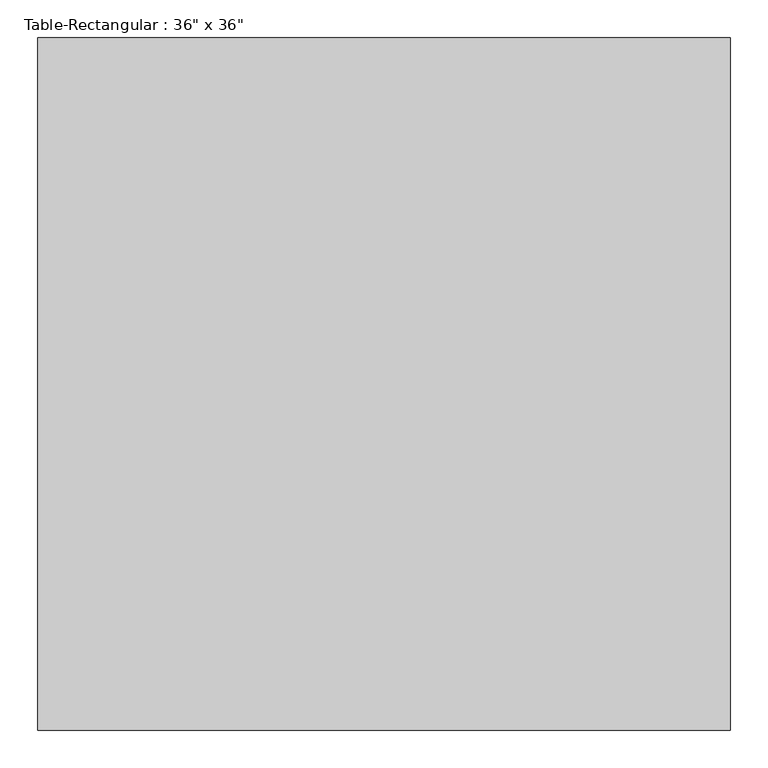
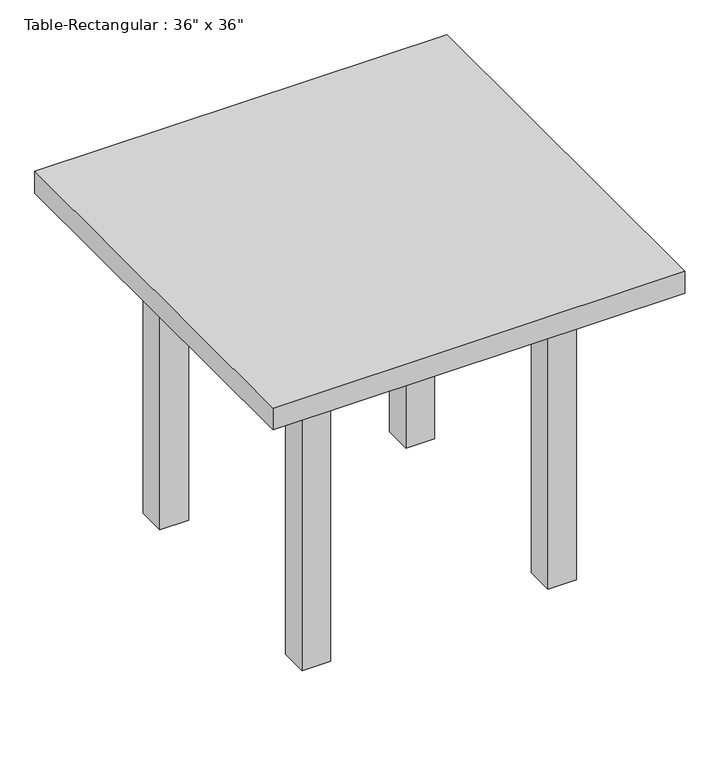
"""IFC4 building model written with IfcOpenShell, lengths in millimetres: furniture geometry."""

from ifc_helpers import new_model, si_unit, frame, origin, origin_with_axes, place, context, project, spatial, polyline, outline, extrude, source, transform, mapped, element, save


def furniture_5106913f(model_context):
    return source(origin(), model_context, "Body", "SweptSolid", [
        extrude(outline(polyline([(-241.3, 304.8), (-241.3, 241.3), (-304.8, 241.3), (-304.8, 304.8), (-241.3, 304.8)])), origin_with_axes(), (0.0, 0.0, 1.0), 711.2),
        extrude(outline(polyline([(241.3, 304.8), (304.8, 304.8), (304.8, 241.3), (241.3, 241.3), (241.3, 304.8)])), origin_with_axes(), (0.0, 0.0, 1.0), 711.2),
        extrude(outline(polyline([(-241.3, -304.8), (-304.8, -304.8), (-304.8, -241.3), (-241.3, -241.3), (-241.3, -304.8)])), origin_with_axes(), (0.0, 0.0, 1.0), 711.2),
        extrude(outline(polyline([(241.3, -304.8), (241.3, -241.3), (304.8, -241.3), (304.8, -304.8), (241.3, -304.8)])), origin_with_axes(), (0.0, 0.0, 1.0), 711.2),
        extrude(outline(polyline([(457.2, 457.2), (457.2, -457.2), (-457.2, -457.2), (-457.2, 457.2), (457.2, 457.2)])), frame((0.0, 0.0, 711.2), z_axis=(0.0, 0.0, 1.0), x_axis=(1.0, 0.0, 0.0)), (0.0, 0.0, 1.0), 50.8),
        extrude(outline(polyline([(241.3, 266.7), (241.3, 241.3), (-241.3, 241.3), (-241.3, 266.7), (241.3, 266.7)])), frame((0.0, 0.0, 609.6), z_axis=(0.0, 0.0, 1.0), x_axis=(1.0, 0.0, 0.0)), (0.0, 0.0, 1.0), 101.6),
        extrude(outline(polyline([(241.3, -266.7), (-241.3, -266.7), (-241.3, -241.3), (241.3, -241.3), (241.3, -266.7)])), frame((0.0, 0.0, 609.6), z_axis=(0.0, 0.0, 1.0), x_axis=(1.0, 0.0, 0.0)), (0.0, 0.0, 1.0), 101.6),
        extrude(outline(polyline([(-254.0, -241.3), (-279.4, -241.3), (-279.4, 241.3), (-254.0, 241.3), (-254.0, -241.3)])), frame((0.0, 0.0, 609.6), z_axis=(0.0, 0.0, 1.0), x_axis=(1.0, 0.0, 0.0)), (0.0, 0.0, 1.0), 101.6),
        extrude(outline(polyline([(254.0, -241.3), (254.0, 241.3), (279.4, 241.3), (279.4, -241.3), (254.0, -241.3)])), frame((0.0, 0.0, 609.6), z_axis=(0.0, 0.0, 1.0), x_axis=(1.0, 0.0, 0.0)), (0.0, 0.0, 1.0), 101.6),
    ])


if __name__ == "__main__":
    model = new_model("IFC4")
    model_context = context("Model", 3, world=origin())
    ifc_project = project(units=[si_unit("LENGTHUNIT", "METRE", prefix="MILLI")], contexts=[model_context])
    site = spatial("IfcSite", under=ifc_project)
    building = spatial("IfcBuilding", under=site)
    placement = place(None, origin())
    furniture_shape = furniture_5106913f(model_context)
    element("IfcFurniture", 1, ObjectType="Table-Rectangular : 36\" x 36\"", at=placement, inside=building, context=model_context, shape_type="MappedRepresentation", body=[
        mapped(furniture_shape, transform((0.0, 0.0, 0.0), x_axis=(1.0, 0.0, 0.0), y_axis=(0.0, 1.0, 0.0), z_axis=(0.0, 0.0, 1.0))),
    ])
    save(model, "model.ifc")

# Revit data of these elements
# Type "Table-Rectangular : 36\" x 36\""
#   Assembly Code = "E2020200"
#   Height = 2' - 6"
#   Length = 3' - 0"
#   Width = 3' - 0"
#   Base Material = Birch
#   Top Material = Birch
#   Default Elevation = 0
# Element 1 (IfcFurniture, "Table-Rectangular : 36\" x 36\"")
#   Materials on its faces: "Birch"
# Materials
#   "Birch": class "Wood", colour RGB 224 178 126, transparency 0, Description = "Betula Alleghaniensis", Cost = 0
